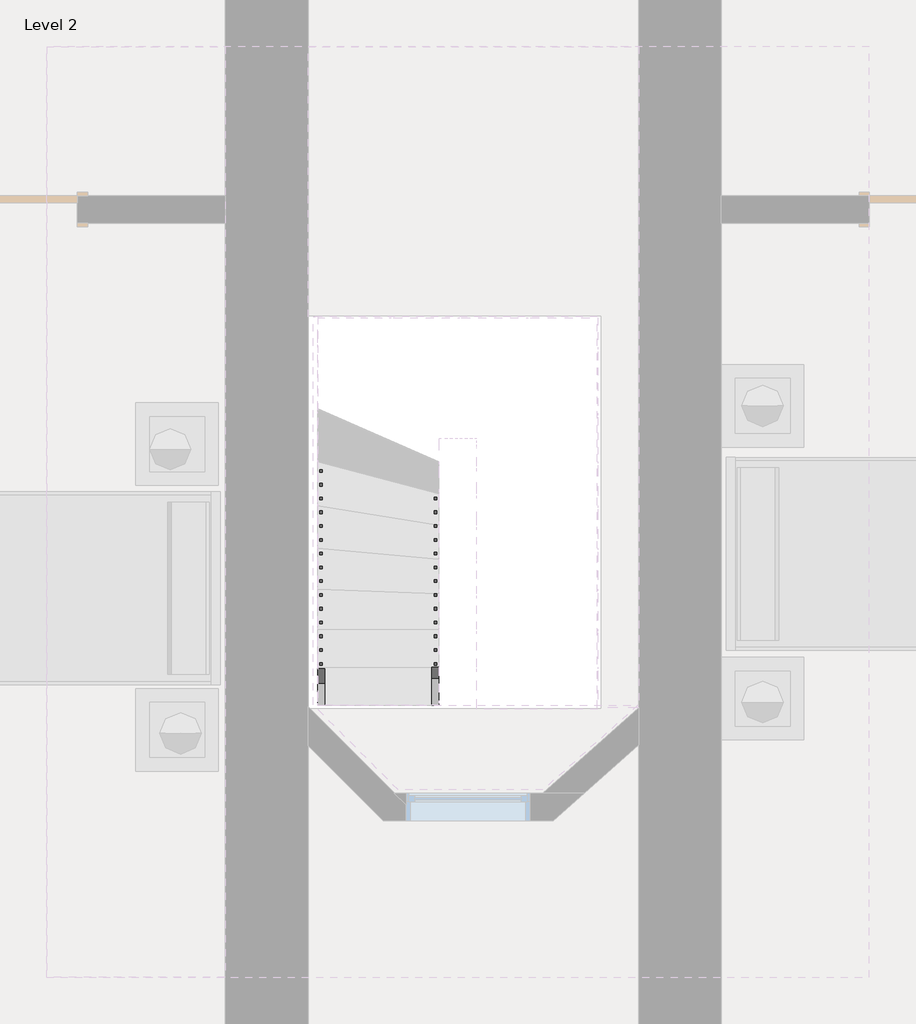
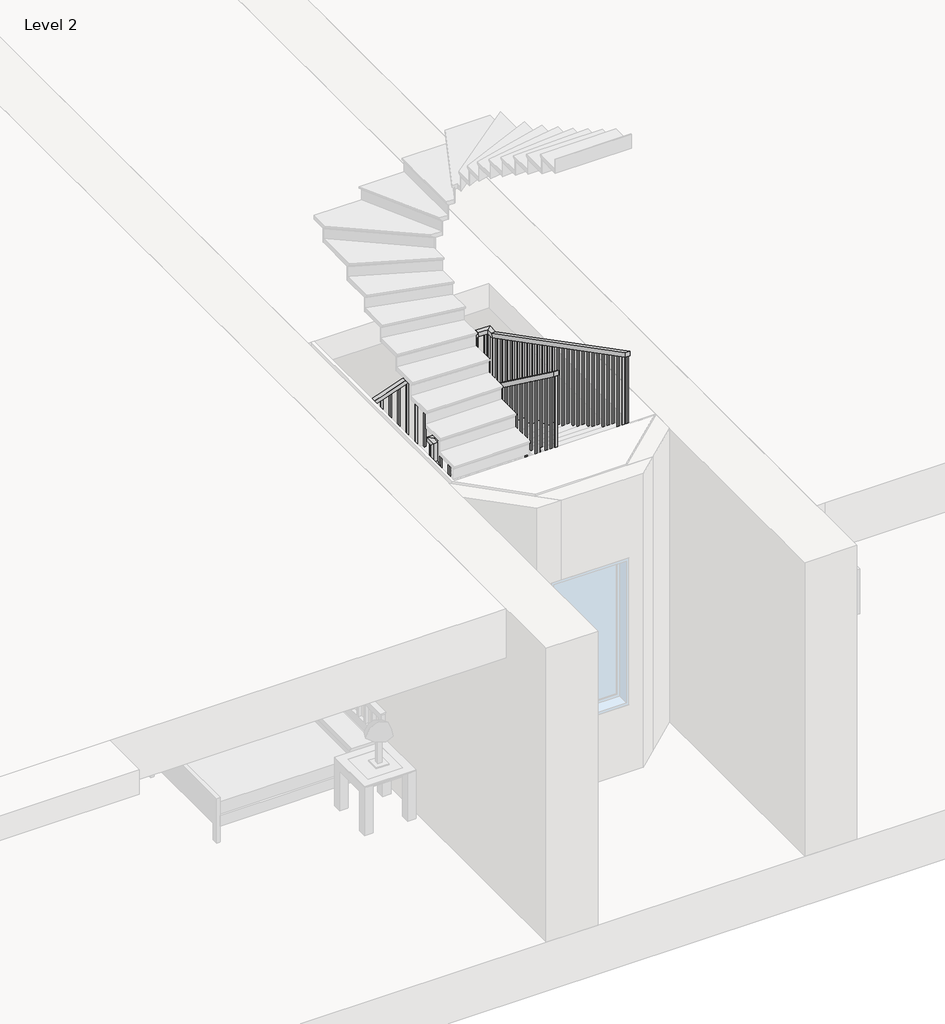
# One storey, part 4 of 5: 2 railings.
"""IFC4 building model written with IfcOpenShell, lengths in millimetres."""

from ifc_helpers import new_model, si_unit, frame, origin, place, context, project, spatial, polyline, outline, extrude, faceted_brep, element, save

model = new_model("IFC4")

# Units and contexts
model_context = context("Model", 3, world=origin())
ifc_project = project(units=[si_unit("LENGTHUNIT", "METRE", prefix="MILLI")], contexts=[model_context])

# Site, building, storey
site = spatial("IfcSite", under=ifc_project)
building = spatial("IfcBuilding", under=site)
storey = spatial("IfcBuildingStorey", under=building, Name="Level 2", Elevation=3657.6)

# Railings
placement = place(None, origin())
element("IfcRailing", 1, ObjectType="Handrail - Rectangular", at=placement, inside=storey, context=model_context, shape_type="SolidModel", body=[
    faceted_brep([(-5097.9987704, -4554.2130548, 4714.7238292), (-5097.9987704, -4554.2130548, 4651.6500708), (-5047.1987704, -4554.2130548, 4651.6500708), (-5047.1987704, -4554.2130548, 4714.7238292), (-5097.9987704, -2667.0424524, 6103.5505468), (-5097.9987704, -2616.2424524, 6077.8620662), (-5047.1987704, -2616.2424524, 6077.8620662), (-5047.1987704, -2667.0424524, 6103.5505468), (-5097.9987704, -2667.0424524, 6336.5326223), (-5097.9987704, -2616.2424524, 6285.7326223), (-5047.1987704, -2616.2424524, 6285.7326223), (-5047.1987704, -2667.0424524, 6336.5326223), (-5097.9987704, -2540.0424524, 6336.5326223), (-5097.9987704, -2540.0424524, 6285.7326223), (-5047.1987704, -2590.8424524, 6285.7326223), (-5047.1987704, -2590.8424524, 6336.5326223), (-4970.9987704, -2540.0424524, 6336.5326223), (-4937.2220362, -2540.0424524, 6285.7326223), (-4937.2220362, -2590.8424524, 6285.7326223), (-4970.9987704, -2590.8424524, 6336.5326223), (-4767.7987704, -2540.0424524, 6820.8625168), (-4767.7987704, -2590.8424524, 6820.8625168), (-4767.7987704, -2590.8424524, 6689.5552229), (-4767.7987704, -2540.0424524, 6689.5552229)], [[[0, 1, 2, 3]], [[1, 0, 4, 5]], [[2, 1, 5, 6]], [[3, 2, 6, 7]], [[0, 3, 7, 4]], [[5, 4, 8, 9]], [[6, 5, 9, 10]], [[7, 6, 10, 11]], [[4, 7, 11, 8]], [[9, 8, 12, 13]], [[10, 9, 13, 14]], [[11, 10, 14, 15]], [[8, 11, 15, 12]], [[13, 12, 16, 17]], [[14, 13, 17, 18]], [[15, 14, 18, 19]], [[12, 15, 19, 16]], [[20, 21, 22, 23]], [[17, 16, 20, 23]], [[18, 17, 23, 22]], [[19, 18, 22, 21]], [[16, 19, 21, 20]]]),
    faceted_brep([(-4716.9987704, -2540.0424524, 6839.4270399), (-4716.9987704, -2540.0424524, 6788.6270399), (-4767.7987704, -2540.0424524, 6788.6270399), (-4767.7987704, -2540.0424524, 6839.4270399), (-4716.9987704, -2622.481404, 6839.4270399), (-4716.9987704, -2639.1592773, 6788.6270399), (-4767.7987704, -2639.1592773, 6788.6270399), (-4767.7987704, -2622.481404, 6839.4270399), (-4716.9987704, -4554.2130546, 8261.0475994), (-4767.7987704, -4554.2130546, 8261.0475994), (-4767.7987704, -4554.2130546, 8197.973841), (-4716.9987704, -4554.2130546, 8197.973841)], [[[0, 1, 2, 3]], [[1, 0, 4, 5]], [[2, 1, 5, 6]], [[3, 2, 6, 7]], [[0, 3, 7, 4]], [[8, 9, 10, 11]], [[5, 4, 8, 11]], [[6, 5, 11, 10]], [[7, 6, 10, 9]], [[4, 7, 9, 8]]]),
    extrude(outline(polyline([(-4562.406404, 8204.0035782), (-4543.356404, 8189.984099), (-4543.356404, 7141.0285714), (-4562.406404, 7141.0285714), (-4562.406404, 8204.0035782)])), frame((-4751.9237704, 0.0, 0.0), z_axis=(1.0, 0.0, 0.0), x_axis=(0.0, 1.0, 0.0)), (0.0, 0.0, 1.0), 19.05),
    extrude(outline(polyline([(-4460.806404, 8129.2330225), (-4441.756404, 8115.2135433), (-4441.756404, 7141.0285714), (-4460.806404, 7141.0285714), (-4460.806404, 8129.2330225)])), frame((-4751.9237704, 0.0, 0.0), z_axis=(1.0, 0.0, 0.0), x_axis=(0.0, 1.0, 0.0)), (0.0, 0.0, 1.0), 19.05),
    extrude(outline(polyline([(-4359.206404, 8054.4624669), (-4340.156404, 8040.4429877), (-4340.156404, 7141.0285714), (-4359.206404, 7141.0285714), (-4359.206404, 8054.4624669)])), frame((-4751.9237704, 0.0, 0.0), z_axis=(1.0, 0.0, 0.0), x_axis=(0.0, 1.0, 0.0)), (0.0, 0.0, 1.0), 19.05),
    extrude(outline(polyline([(-4257.606404, 7979.6919113), (-4238.556404, 7965.6724321), (-4238.556404, 6966.8571429), (-4257.606404, 6966.8571429), (-4257.606404, 7979.6919113)])), frame((-4751.9237704, 0.0, 0.0), z_axis=(1.0, 0.0, 0.0), x_axis=(0.0, 1.0, 0.0)), (0.0, 0.0, 1.0), 19.05),
    extrude(outline(polyline([(-4156.006404, 7904.9213556), (-4136.956404, 7890.9018764), (-4136.956404, 6966.8571429), (-4156.006404, 6966.8571429), (-4156.006404, 7904.9213556)])), frame((-4751.9237704, 0.0, 0.0), z_axis=(1.0, 0.0, 0.0), x_axis=(0.0, 1.0, 0.0)), (0.0, 0.0, 1.0), 19.05),
    extrude(outline(polyline([(-4054.406404, 7830.1508), (-4035.356404, 7816.1313208), (-4035.356404, 6966.8571429), (-4054.406404, 6966.8571429), (-4054.406404, 7830.1508)])), frame((-4751.9237704, 0.0, 0.0), z_axis=(1.0, 0.0, 0.0), x_axis=(0.0, 1.0, 0.0)), (0.0, 0.0, 1.0), 19.05),
    extrude(outline(polyline([(-3952.806404, 7755.3802444), (-3933.756404, 7741.3607652), (-3933.756404, 6792.6857143), (-3952.806404, 6792.6857143), (-3952.806404, 7755.3802444)])), frame((-4751.9237704, 0.0, 0.0), z_axis=(1.0, 0.0, 0.0), x_axis=(0.0, 1.0, 0.0)), (0.0, 0.0, 1.0), 19.05),
    extrude(outline(polyline([(-3851.206404, 7680.6096887), (-3832.156404, 7666.5902095), (-3832.156404, 6792.6857143), (-3851.206404, 6792.6857143), (-3851.206404, 7680.6096887)])), frame((-4751.9237704, 0.0, 0.0), z_axis=(1.0, 0.0, 0.0), x_axis=(0.0, 1.0, 0.0)), (0.0, 0.0, 1.0), 19.05),
    extrude(outline(polyline([(-3749.606404, 7605.8391331), (-3730.556404, 7591.8196539), (-3730.556404, 6792.6857143), (-3749.606404, 6792.6857143), (-3749.606404, 7605.8391331)])), frame((-4751.9237704, 0.0, 0.0), z_axis=(1.0, 0.0, 0.0), x_axis=(0.0, 1.0, 0.0)), (0.0, 0.0, 1.0), 19.05),
    extrude(outline(polyline([(-3648.006404, 7531.0685775), (-3628.956404, 7517.0490983), (-3628.956404, 6618.5142857), (-3648.006404, 6618.5142857), (-3648.006404, 7531.0685775)])), frame((-4751.9237704, 0.0, 0.0), z_axis=(1.0, 0.0, 0.0), x_axis=(0.0, 1.0, 0.0)), (0.0, 0.0, 1.0), 19.05),
    extrude(outline(polyline([(-3546.406404, 7456.2980218), (-3527.356404, 7442.2785426), (-3527.356404, 6618.5142857), (-3546.406404, 6618.5142857), (-3546.406404, 7456.2980218)])), frame((-4751.9237704, 0.0, 0.0), z_axis=(1.0, 0.0, 0.0), x_axis=(0.0, 1.0, 0.0)), (0.0, 0.0, 1.0), 19.05),
    extrude(outline(polyline([(-3444.806404, 7381.5274662), (-3425.756404, 7367.507987), (-3425.756404, 6444.3428571), (-3444.806404, 6444.3428571), (-3444.806404, 7381.5274662)])), frame((-4751.9237704, 0.0, 0.0), z_axis=(1.0, 0.0, 0.0), x_axis=(0.0, 1.0, 0.0)), (0.0, 0.0, 1.0), 19.05),
    extrude(outline(polyline([(-3343.206404, 7306.7569106), (-3324.156404, 7292.7374314), (-3324.156404, 6444.3428571), (-3343.206404, 6444.3428571), (-3343.206404, 7306.7569106)])), frame((-4751.9237704, 0.0, 0.0), z_axis=(1.0, 0.0, 0.0), x_axis=(0.0, 1.0, 0.0)), (0.0, 0.0, 1.0), 19.05),
    extrude(outline(polyline([(-3241.606404, 7231.9863549), (-3222.556404, 7217.9668757), (-3222.556404, 6444.3428571), (-3241.606404, 6444.3428571), (-3241.606404, 7231.9863549)])), frame((-4751.9237704, 0.0, 0.0), z_axis=(1.0, 0.0, 0.0), x_axis=(0.0, 1.0, 0.0)), (0.0, 0.0, 1.0), 19.05),
    extrude(outline(polyline([(-3140.006404, 7157.2157993), (-3120.956404, 7143.1963201), (-3120.956404, 6270.1714286), (-3140.006404, 6270.1714286), (-3140.006404, 7157.2157993)])), frame((-4751.9237704, 0.0, 0.0), z_axis=(1.0, 0.0, 0.0), x_axis=(0.0, 1.0, 0.0)), (0.0, 0.0, 1.0), 19.05),
    extrude(outline(polyline([(-3038.406404, 7082.4452436), (-3019.356404, 7068.4257645), (-3019.356404, 6270.1714286), (-3038.406404, 6270.1714286), (-3038.406404, 7082.4452436)])), frame((-4751.9237704, 0.0, 0.0), z_axis=(1.0, 0.0, 0.0), x_axis=(0.0, 1.0, 0.0)), (0.0, 0.0, 1.0), 19.05),
    extrude(outline(polyline([(-2936.806404, 7007.674688), (-2917.756404, 6993.6552088), (-2917.756404, 6096.0), (-2936.806404, 6096.0), (-2936.806404, 7007.674688)])), frame((-4751.9237704, 0.0, 0.0), z_axis=(1.0, 0.0, 0.0), x_axis=(0.0, 1.0, 0.0)), (0.0, 0.0, 1.0), 19.05),
    extrude(outline(polyline([(-2835.206404, 6932.9041324), (-2816.156404, 6918.8846532), (-2816.156404, 6096.0), (-2835.206404, 6096.0), (-2835.206404, 6932.9041324)])), frame((-4751.9237704, 0.0, 0.0), z_axis=(1.0, 0.0, 0.0), x_axis=(0.0, 1.0, 0.0)), (0.0, 0.0, 1.0), 19.05),
    extrude(outline(polyline([(-2733.606404, 6858.1335767), (-2714.556404, 6844.1140976), (-2714.556404, 5921.8285714), (-2733.606404, 5921.8285714), (-2733.606404, 6858.1335767)])), frame((-4751.9237704, 0.0, 0.0), z_axis=(1.0, 0.0, 0.0), x_axis=(0.0, 1.0, 0.0)), (0.0, 0.0, 1.0), 19.05),
    extrude(outline(polyline([(6512.0699532, -4842.2624928), (6466.6640255, -4861.3124928), (5573.4857143, -4861.3124928), (5573.4857143, -4842.2624928), (6512.0699532, -4842.2624928)])), frame((0.0, -2574.9674524, 0.0), z_axis=(0.0, 1.0, 0.0), x_axis=(0.0, 0.0, 1.0)), (0.0, 0.0, 1.0), 19.05),
    extrude(outline(polyline([(6269.9050059, -4943.8624928), (6224.4990783, -4962.9124928), (5399.3142857, -4962.9124928), (5399.3142857, -4943.8624928), (6269.9050059, -4943.8624928)])), frame((0.0, -2574.9674524, 0.0), z_axis=(0.0, 1.0, 0.0), x_axis=(0.0, 0.0, 1.0)), (0.0, 0.0, 1.0), 19.05),
    extrude(outline(polyline([(-2633.3380548, 6065.2808881), (-2614.2880548, 6079.3003673), (-2614.2880548, 5050.9714286), (-2633.3380548, 5050.9714286), (-2633.3380548, 6065.2808881)])), frame((-5082.1237704, 0.0, 0.0), z_axis=(1.0, 0.0, 0.0), x_axis=(0.0, 1.0, 0.0)), (0.0, 0.0, 1.0), 19.05),
    extrude(outline(polyline([(-2734.9380548, 5990.5103325), (-2715.8880548, 6004.5298117), (-2715.8880548, 5050.9714286), (-2734.9380548, 5050.9714286), (-2734.9380548, 5990.5103325)])), frame((-5082.1237704, 0.0, 0.0), z_axis=(1.0, 0.0, 0.0), x_axis=(0.0, 1.0, 0.0)), (0.0, 0.0, 1.0), 19.05),
    extrude(outline(polyline([(-2836.5380548, 5915.7397768), (-2817.4880548, 5929.759256), (-2817.4880548, 4876.8), (-2836.5380548, 4876.8), (-2836.5380548, 5915.7397768)])), frame((-5082.1237704, 0.0, 0.0), z_axis=(1.0, 0.0, 0.0), x_axis=(0.0, 1.0, 0.0)), (0.0, 0.0, 1.0), 19.05),
    extrude(outline(polyline([(-2938.1380548, 5840.9692212), (-2919.0880548, 5854.9887004), (-2919.0880548, 4876.8), (-2938.1380548, 4876.8), (-2938.1380548, 5840.9692212)])), frame((-5082.1237704, 0.0, 0.0), z_axis=(1.0, 0.0, 0.0), x_axis=(0.0, 1.0, 0.0)), (0.0, 0.0, 1.0), 19.05),
    extrude(outline(polyline([(-3039.7380548, 5766.1986656), (-3020.6880548, 5780.2181448), (-3020.6880548, 4702.6285714), (-3039.7380548, 4702.6285714), (-3039.7380548, 5766.1986656)])), frame((-5082.1237704, 0.0, 0.0), z_axis=(1.0, 0.0, 0.0), x_axis=(0.0, 1.0, 0.0)), (0.0, 0.0, 1.0), 19.05),
    extrude(outline(polyline([(-3141.3380548, 5691.42811), (-3122.2880548, 5705.4475891), (-3122.2880548, 4702.6285714), (-3141.3380548, 4702.6285714), (-3141.3380548, 5691.42811)])), frame((-5082.1237704, 0.0, 0.0), z_axis=(1.0, 0.0, 0.0), x_axis=(0.0, 1.0, 0.0)), (0.0, 0.0, 1.0), 19.05),
    extrude(outline(polyline([(-3242.9380548, 5616.6575543), (-3223.8880548, 5630.6770335), (-3223.8880548, 4528.4571429), (-3242.9380548, 4528.4571429), (-3242.9380548, 5616.6575543)])), frame((-5082.1237704, 0.0, 0.0), z_axis=(1.0, 0.0, 0.0), x_axis=(0.0, 1.0, 0.0)), (0.0, 0.0, 1.0), 19.05),
    extrude(outline(polyline([(-3344.5380548, 5541.8869987), (-3325.4880548, 5555.9064779), (-3325.4880548, 4528.4571429), (-3344.5380548, 4528.4571429), (-3344.5380548, 5541.8869987)])), frame((-5082.1237704, 0.0, 0.0), z_axis=(1.0, 0.0, 0.0), x_axis=(0.0, 1.0, 0.0)), (0.0, 0.0, 1.0), 19.05),
    extrude(outline(polyline([(-3446.1380548, 5467.1164431), (-3427.0880548, 5481.1359223), (-3427.0880548, 4528.4571429), (-3446.1380548, 4528.4571429), (-3446.1380548, 5467.1164431)])), frame((-5082.1237704, 0.0, 0.0), z_axis=(1.0, 0.0, 0.0), x_axis=(0.0, 1.0, 0.0)), (0.0, 0.0, 1.0), 19.05),
    extrude(outline(polyline([(-3547.7380548, 5392.3458875), (-3528.6880548, 5406.3653666), (-3528.6880548, 4354.2857143), (-3547.7380548, 4354.2857143), (-3547.7380548, 5392.3458875)])), frame((-5082.1237704, 0.0, 0.0), z_axis=(1.0, 0.0, 0.0), x_axis=(0.0, 1.0, 0.0)), (0.0, 0.0, 1.0), 19.05),
    extrude(outline(polyline([(-3649.3380548, 5317.5753318), (-3630.2880548, 5331.594811), (-3630.2880548, 4354.2857143), (-3649.3380548, 4354.2857143), (-3649.3380548, 5317.5753318)])), frame((-5082.1237704, 0.0, 0.0), z_axis=(1.0, 0.0, 0.0), x_axis=(0.0, 1.0, 0.0)), (0.0, 0.0, 1.0), 19.05),
    extrude(outline(polyline([(-3750.9380548, 5242.8047762), (-3731.8880548, 5256.8242554), (-3731.8880548, 4180.1142857), (-3750.9380548, 4180.1142857), (-3750.9380548, 5242.8047762)])), frame((-5082.1237704, 0.0, 0.0), z_axis=(1.0, 0.0, 0.0), x_axis=(0.0, 1.0, 0.0)), (0.0, 0.0, 1.0), 19.05),
    extrude(outline(polyline([(-3852.5380548, 5168.0342206), (-3833.4880548, 5182.0536998), (-3833.4880548, 4180.1142857), (-3852.5380548, 4180.1142857), (-3852.5380548, 5168.0342206)])), frame((-5082.1237704, 0.0, 0.0), z_axis=(1.0, 0.0, 0.0), x_axis=(0.0, 1.0, 0.0)), (0.0, 0.0, 1.0), 19.05),
    extrude(outline(polyline([(-3954.1380548, 5093.263665), (-3935.0880548, 5107.2831441), (-3935.0880548, 4180.1142857), (-3954.1380548, 4180.1142857), (-3954.1380548, 5093.263665)])), frame((-5082.1237704, 0.0, 0.0), z_axis=(1.0, 0.0, 0.0), x_axis=(0.0, 1.0, 0.0)), (0.0, 0.0, 1.0), 19.05),
    extrude(outline(polyline([(-4055.7380548, 5018.4931093), (-4036.6880548, 5032.5125885), (-4036.6880548, 4005.9428571), (-4055.7380548, 4005.9428571), (-4055.7380548, 5018.4931093)])), frame((-5082.1237704, 0.0, 0.0), z_axis=(1.0, 0.0, 0.0), x_axis=(0.0, 1.0, 0.0)), (0.0, 0.0, 1.0), 19.05),
    extrude(outline(polyline([(-4157.3380548, 4943.7225537), (-4138.2880548, 4957.7420329), (-4138.2880548, 4005.9428571), (-4157.3380548, 4005.9428571), (-4157.3380548, 4943.7225537)])), frame((-5082.1237704, 0.0, 0.0), z_axis=(1.0, 0.0, 0.0), x_axis=(0.0, 1.0, 0.0)), (0.0, 0.0, 1.0), 19.05),
    extrude(outline(polyline([(-4258.9380548, 4868.9519981), (-4239.8880548, 4882.9714773), (-4239.8880548, 4005.9428571), (-4258.9380548, 4005.9428571), (-4258.9380548, 4868.9519981)])), frame((-5082.1237704, 0.0, 0.0), z_axis=(1.0, 0.0, 0.0), x_axis=(0.0, 1.0, 0.0)), (0.0, 0.0, 1.0), 19.05),
    extrude(outline(polyline([(-4360.5380548, 4794.1814424), (-4341.4880548, 4808.2009216), (-4341.4880548, 3831.7714286), (-4360.5380548, 3831.7714286), (-4360.5380548, 4794.1814424)])), frame((-5082.1237704, 0.0, 0.0), z_axis=(1.0, 0.0, 0.0), x_axis=(0.0, 1.0, 0.0)), (0.0, 0.0, 1.0), 19.05),
    extrude(outline(polyline([(-4462.1380548, 4719.4108868), (-4443.0880548, 4733.430366), (-4443.0880548, 3831.7714286), (-4462.1380548, 3831.7714286), (-4462.1380548, 4719.4108868)])), frame((-5082.1237704, 0.0, 0.0), z_axis=(1.0, 0.0, 0.0), x_axis=(0.0, 1.0, 0.0)), (0.0, 0.0, 1.0), 19.05),
    extrude(outline(polyline([(-4751.9237704, -2612.956404), (-4732.8737704, -2612.956404), (-4732.8737704, -2632.006404), (-4751.9237704, -2632.006404), (-4751.9237704, -2612.956404)])), frame((0.0, 0.0, 5921.8285714), z_axis=(0.0, 0.0, 1.0), x_axis=(1.0, 0.0, 0.0)), (0.0, 0.0, 1.0), 866.7984685),
    extrude(outline(polyline([(6772.7994235, -4732.8737704), (6727.3934959, -4751.9237704), (5747.6571429, -4751.9237704), (5747.6571429, -4732.8737704), (6772.7994235, -4732.8737704)])), frame((0.0, -2574.9674524, 0.0), z_axis=(0.0, 1.0, 0.0), x_axis=(0.0, 0.0, 1.0)), (0.0, 0.0, 1.0), 19.05),
    extrude(outline(polyline([(6730.8227099, -4750.485048), (6685.4167823, -4769.535048), (5747.6571429, -4769.535048), (5747.6571429, -4750.485048), (6730.8227099, -4750.485048)])), frame((0.0, -2574.9674524, 0.0), z_axis=(0.0, 1.0, 0.0), x_axis=(0.0, 0.0, 1.0)), (0.0, 0.0, 1.0), 19.05),
    extrude(outline(polyline([(-5064.5124928, -2574.9674524), (-5064.5124928, -2555.9174524), (-5045.4624928, -2555.9174524), (-5045.4624928, -2574.9674524), (-5064.5124928, -2574.9674524)])), frame((0.0, 0.0, 5225.1428571), z_axis=(0.0, 0.0, 1.0), x_axis=(1.0, 0.0, 0.0)), (0.0, 0.0, 1.0), 1060.5897652),
    extrude(outline(polyline([(-5063.0737704, -2574.9674524), (-5082.1237704, -2574.9674524), (-5082.1237704, -2555.9174524), (-5063.0737704, -2555.9174524), (-5063.0737704, -2574.9674524)])), frame((0.0, 0.0, 5225.1428571), z_axis=(0.0, 0.0, 1.0), x_axis=(1.0, 0.0, 0.0)), (0.0, 0.0, 1.0), 1060.5897652),
    extrude(outline(polyline([(-2632.006404, 6066.2608908), (-2612.956404, 6080.2803699), (-2612.956404, 5050.9714286), (-2632.006404, 5050.9714286), (-2632.006404, 6066.2608908)])), frame((-5082.1237704, 0.0, 0.0), z_axis=(1.0, 0.0, 0.0), x_axis=(0.0, 1.0, 0.0)), (0.0, 0.0, 1.0), 19.05),
    extrude(outline(polyline([(-4554.2130546, 8197.973841), (-4535.1630546, 8183.9543619), (-4535.1630546, 7141.0285714), (-4554.2130546, 7141.0285714), (-4554.2130546, 8197.973841)])), frame((-4751.9237704, 0.0, 0.0), z_axis=(1.0, 0.0, 0.0), x_axis=(0.0, 1.0, 0.0)), (0.0, 0.0, 1.0), 19.05),
    extrude(outline(polyline([(-4554.2130548, 4651.6500708), (-4535.1630548, 4665.66955), (-4535.1630548, 3831.7714286), (-4554.2130548, 3831.7714286), (-4554.2130548, 4651.6500708)])), frame((-5082.1237704, 0.0, 0.0), z_axis=(1.0, 0.0, 0.0), x_axis=(0.0, 1.0, 0.0)), (0.0, 0.0, 1.0), 19.05),
])
element("IfcRailing", 2, ObjectType="Handrail - Rectangular", at=placement, inside=storey, context=model_context, shape_type="SolidModel", body=[
    faceted_brep([(-5940.8822214, -4554.2130548, 4776.0197691), (-5940.8822214, -4554.2130548, 4718.8427889), (-5890.0822214, -4554.2130548, 4718.8427889), (-5890.0822214, -4554.2130548, 4776.0197691), (-5940.8822214, -1817.6237991, 6189.5953311), (-5940.8822214, -1805.2783851, 6138.7953311), (-5890.0822214, -1805.2783851, 6138.7953311), (-5890.0822214, -1817.6237991, 6189.5953311), (-5940.8822214, -1697.1590014, 6189.5953311), (-5940.8822214, -1697.1590014, 6138.7953311), (-5890.0822214, -1747.9590014, 6138.7953311), (-5890.0822214, -1747.9590014, 6189.5953311), (-5773.0008737, -1697.1590014, 6189.5953311), (-5764.4924766, -1697.1590014, 6138.7953311), (-5764.4924766, -1747.9590014, 6138.7953311), (-5773.0008737, -1747.9590014, 6189.5953311), (-4041.9966669, -1697.1590014, 6786.1760978), (-4033.4882698, -1697.1590014, 6735.3760978), (-4033.4882698, -1747.9590014, 6735.3760978), (-4041.9966669, -1747.9590014, 6786.1760978), (-3874.1153195, -1697.1590014, 6786.1760978), (-3874.1153195, -1697.1590014, 6735.3760978), (-3924.9153195, -1747.9590014, 6735.3760978), (-3924.9153195, -1747.9590014, 6786.1760978), (-3874.1153195, -1817.6237989, 6786.1760978), (-3874.1153195, -1829.9692129, 6735.3760978), (-3924.9153195, -1829.9692129, 6735.3760978), (-3924.9153195, -1817.6237989, 6786.1760978), (-3874.1153195, -4554.2130546, 8199.7516594), (-3924.9153195, -4554.2130546, 8199.7516594), (-3924.9153195, -4554.2130546, 8142.5746792), (-3874.1153195, -4554.2130546, 8142.5746792)], [[[0, 1, 2, 3]], [[1, 0, 4, 5]], [[2, 1, 5, 6]], [[3, 2, 6, 7]], [[0, 3, 7, 4]], [[5, 4, 8, 9]], [[6, 5, 9, 10]], [[7, 6, 10, 11]], [[4, 7, 11, 8]], [[9, 8, 12, 13]], [[10, 9, 13, 14]], [[11, 10, 14, 15]], [[8, 11, 15, 12]], [[13, 12, 16, 17]], [[14, 13, 17, 18]], [[15, 14, 18, 19]], [[12, 15, 19, 16]], [[17, 16, 20, 21]], [[18, 17, 21, 22]], [[19, 18, 22, 23]], [[16, 19, 23, 20]], [[21, 20, 24, 25]], [[22, 21, 25, 26]], [[23, 22, 26, 27]], [[20, 23, 27, 24]], [[28, 29, 30, 31]], [[25, 24, 28, 31]], [[26, 25, 31, 30]], [[27, 26, 30, 29]], [[24, 27, 29, 28]]]),
    extrude(outline(polyline([(-4449.6987989, 8088.5882078), (-4449.6987989, 7141.0285714), (-4468.7487989, 7141.0285714), (-4468.7487989, 8098.4284183), (-4449.6987989, 8088.5882078)])), frame((-3909.0403195, 0.0, 0.0), z_axis=(1.0, 0.0, 0.0), x_axis=(0.0, 1.0, 0.0)), (0.0, 0.0, 1.0), 19.05),
    extrude(outline(polyline([(-4348.0987989, 8036.1070849), (-4348.0987989, 7141.0285714), (-4367.1487989, 7141.0285714), (-4367.1487989, 8045.9472954), (-4348.0987989, 8036.1070849)])), frame((-3909.0403195, 0.0, 0.0), z_axis=(1.0, 0.0, 0.0), x_axis=(0.0, 1.0, 0.0)), (0.0, 0.0, 1.0), 19.05),
    extrude(outline(polyline([(-4246.4987989, 7983.625962), (-4246.4987989, 6966.8571429), (-4265.5487989, 6966.8571429), (-4265.5487989, 7993.4661725), (-4246.4987989, 7983.625962)])), frame((-3909.0403195, 0.0, 0.0), z_axis=(1.0, 0.0, 0.0), x_axis=(0.0, 1.0, 0.0)), (0.0, 0.0, 1.0), 19.05),
    extrude(outline(polyline([(-4144.8987989, 7931.1448391), (-4144.8987989, 6966.8571429), (-4163.9487989, 6966.8571429), (-4163.9487989, 7940.9850496), (-4144.8987989, 7931.1448391)])), frame((-3909.0403195, 0.0, 0.0), z_axis=(1.0, 0.0, 0.0), x_axis=(0.0, 1.0, 0.0)), (0.0, 0.0, 1.0), 19.05),
    extrude(outline(polyline([(-4043.2987989, 7878.6637162), (-4043.2987989, 6966.8571429), (-4062.3487989, 6966.8571429), (-4062.3487989, 7888.5039267), (-4043.2987989, 7878.6637162)])), frame((-3909.0403195, 0.0, 0.0), z_axis=(1.0, 0.0, 0.0), x_axis=(0.0, 1.0, 0.0)), (0.0, 0.0, 1.0), 19.05),
    extrude(outline(polyline([(-3941.6987989, 7826.1825933), (-3941.6987989, 6792.6857143), (-3960.7487989, 6792.6857143), (-3960.7487989, 7836.0228038), (-3941.6987989, 7826.1825933)])), frame((-3909.0403195, 0.0, 0.0), z_axis=(1.0, 0.0, 0.0), x_axis=(0.0, 1.0, 0.0)), (0.0, 0.0, 1.0), 19.05),
    extrude(outline(polyline([(-3840.0987989, 7773.7014704), (-3840.0987989, 6792.6857143), (-3859.1487989, 6792.6857143), (-3859.1487989, 7783.5416809), (-3840.0987989, 7773.7014704)])), frame((-3909.0403195, 0.0, 0.0), z_axis=(1.0, 0.0, 0.0), x_axis=(0.0, 1.0, 0.0)), (0.0, 0.0, 1.0), 19.05),
    extrude(outline(polyline([(-3738.4987989, 7721.2203475), (-3738.4987989, 6792.6857143), (-3757.5487989, 6792.6857143), (-3757.5487989, 7731.060558), (-3738.4987989, 7721.2203475)])), frame((-3909.0403195, 0.0, 0.0), z_axis=(1.0, 0.0, 0.0), x_axis=(0.0, 1.0, 0.0)), (0.0, 0.0, 1.0), 19.05),
    extrude(outline(polyline([(-3636.8987989, 7668.7392246), (-3636.8987989, 6618.5142857), (-3655.9487989, 6618.5142857), (-3655.9487989, 7678.5794351), (-3636.8987989, 7668.7392246)])), frame((-3909.0403195, 0.0, 0.0), z_axis=(1.0, 0.0, 0.0), x_axis=(0.0, 1.0, 0.0)), (0.0, 0.0, 1.0), 19.05),
    extrude(outline(polyline([(-3535.2987989, 7616.2581017), (-3535.2987989, 6618.5142857), (-3554.3487989, 6618.5142857), (-3554.3487989, 7626.0983122), (-3535.2987989, 7616.2581017)])), frame((-3909.0403195, 0.0, 0.0), z_axis=(1.0, 0.0, 0.0), x_axis=(0.0, 1.0, 0.0)), (0.0, 0.0, 1.0), 19.05),
    extrude(outline(polyline([(-3433.6987989, 7563.7769788), (-3433.6987989, 6618.5142857), (-3452.7487989, 6618.5142857), (-3452.7487989, 7573.6171893), (-3433.6987989, 7563.7769788)])), frame((-3909.0403195, 0.0, 0.0), z_axis=(1.0, 0.0, 0.0), x_axis=(0.0, 1.0, 0.0)), (0.0, 0.0, 1.0), 19.05),
    extrude(outline(polyline([(-3332.0987989, 7511.2958559), (-3332.0987989, 6444.3428571), (-3351.1487989, 6444.3428571), (-3351.1487989, 7521.1360664), (-3332.0987989, 7511.2958559)])), frame((-3909.0403195, 0.0, 0.0), z_axis=(1.0, 0.0, 0.0), x_axis=(0.0, 1.0, 0.0)), (0.0, 0.0, 1.0), 19.05),
    extrude(outline(polyline([(-3230.4987989, 7458.814733), (-3230.4987989, 6444.3428571), (-3249.5487989, 6444.3428571), (-3249.5487989, 7468.6549435), (-3230.4987989, 7458.814733)])), frame((-3909.0403195, 0.0, 0.0), z_axis=(1.0, 0.0, 0.0), x_axis=(0.0, 1.0, 0.0)), (0.0, 0.0, 1.0), 19.05),
    extrude(outline(polyline([(-3128.8987989, 7406.33361), (-3128.8987989, 6444.3428571), (-3147.9487989, 6444.3428571), (-3147.9487989, 7416.1738206), (-3128.8987989, 7406.33361)])), frame((-3909.0403195, 0.0, 0.0), z_axis=(1.0, 0.0, 0.0), x_axis=(0.0, 1.0, 0.0)), (0.0, 0.0, 1.0), 19.05),
    extrude(outline(polyline([(-3027.2987989, 7353.8524871), (-3027.2987989, 6270.1714286), (-3046.3487989, 6270.1714286), (-3046.3487989, 7363.6926977), (-3027.2987989, 7353.8524871)])), frame((-3909.0403195, 0.0, 0.0), z_axis=(1.0, 0.0, 0.0), x_axis=(0.0, 1.0, 0.0)), (0.0, 0.0, 1.0), 19.05),
    extrude(outline(polyline([(-2925.6987989, 7301.3713642), (-2925.6987989, 6270.1714286), (-2944.7487989, 6270.1714286), (-2944.7487989, 7311.2115748), (-2925.6987989, 7301.3713642)])), frame((-3909.0403195, 0.0, 0.0), z_axis=(1.0, 0.0, 0.0), x_axis=(0.0, 1.0, 0.0)), (0.0, 0.0, 1.0), 19.05),
    extrude(outline(polyline([(-2824.0987989, 7248.8902413), (-2824.0987989, 6270.1714286), (-2843.1487989, 6270.1714286), (-2843.1487989, 7258.7304519), (-2824.0987989, 7248.8902413)])), frame((-3909.0403195, 0.0, 0.0), z_axis=(1.0, 0.0, 0.0), x_axis=(0.0, 1.0, 0.0)), (0.0, 0.0, 1.0), 19.05),
    extrude(outline(polyline([(-2722.4987989, 7196.4091184), (-2722.4987989, 6096.0), (-2741.5487989, 6096.0), (-2741.5487989, 7206.249329), (-2722.4987989, 7196.4091184)])), frame((-3909.0403195, 0.0, 0.0), z_axis=(1.0, 0.0, 0.0), x_axis=(0.0, 1.0, 0.0)), (0.0, 0.0, 1.0), 19.05),
    extrude(outline(polyline([(-2620.8987989, 7143.9279955), (-2620.8987989, 6096.0), (-2639.9487989, 6096.0), (-2639.9487989, 7153.7682061), (-2620.8987989, 7143.9279955)])), frame((-3909.0403195, 0.0, 0.0), z_axis=(1.0, 0.0, 0.0), x_axis=(0.0, 1.0, 0.0)), (0.0, 0.0, 1.0), 19.05),
    extrude(outline(polyline([(-2519.2987989, 7091.4468726), (-2519.2987989, 6096.0), (-2538.3487989, 6096.0), (-2538.3487989, 7101.2870832), (-2519.2987989, 7091.4468726)])), frame((-3909.0403195, 0.0, 0.0), z_axis=(1.0, 0.0, 0.0), x_axis=(0.0, 1.0, 0.0)), (0.0, 0.0, 1.0), 19.05),
    extrude(outline(polyline([(-2417.6987989, 7038.9657497), (-2417.6987989, 6096.0), (-2436.7487989, 6096.0), (-2436.7487989, 7048.8059603), (-2417.6987989, 7038.9657497)])), frame((-3909.0403195, 0.0, 0.0), z_axis=(1.0, 0.0, 0.0), x_axis=(0.0, 1.0, 0.0)), (0.0, 0.0, 1.0), 19.05),
    extrude(outline(polyline([(-2316.0987989, 6986.4846268), (-2316.0987989, 5921.8285714), (-2335.1487989, 5921.8285714), (-2335.1487989, 6996.3248374), (-2316.0987989, 6986.4846268)])), frame((-3909.0403195, 0.0, 0.0), z_axis=(1.0, 0.0, 0.0), x_axis=(0.0, 1.0, 0.0)), (0.0, 0.0, 1.0), 19.05),
    extrude(outline(polyline([(-2214.4987989, 6934.0035039), (-2214.4987989, 5921.8285714), (-2233.5487989, 5921.8285714), (-2233.5487989, 6943.8437145), (-2214.4987989, 6934.0035039)])), frame((-3909.0403195, 0.0, 0.0), z_axis=(1.0, 0.0, 0.0), x_axis=(0.0, 1.0, 0.0)), (0.0, 0.0, 1.0), 19.05),
    extrude(outline(polyline([(-2112.8987989, 6881.522381), (-2112.8987989, 5921.8285714), (-2131.9487989, 5921.8285714), (-2131.9487989, 6891.3625916), (-2112.8987989, 6881.522381)])), frame((-3909.0403195, 0.0, 0.0), z_axis=(1.0, 0.0, 0.0), x_axis=(0.0, 1.0, 0.0)), (0.0, 0.0, 1.0), 19.05),
    extrude(outline(polyline([(-2011.2987989, 6829.0412581), (-2011.2987989, 5921.8285714), (-2030.3487989, 5921.8285714), (-2030.3487989, 6838.8814687), (-2011.2987989, 6829.0412581)])), frame((-3909.0403195, 0.0, 0.0), z_axis=(1.0, 0.0, 0.0), x_axis=(0.0, 1.0, 0.0)), (0.0, 0.0, 1.0), 19.05),
    extrude(outline(polyline([(-1909.6987989, 6776.5601352), (-1909.6987989, 5747.6571429), (-1928.7487989, 5747.6571429), (-1928.7487989, 6786.4003458), (-1909.6987989, 6776.5601352)])), frame((-3909.0403195, 0.0, 0.0), z_axis=(1.0, 0.0, 0.0), x_axis=(0.0, 1.0, 0.0)), (0.0, 0.0, 1.0), 19.05),
    extrude(outline(polyline([(-3949.9216669, -1713.0340014), (-3930.8716669, -1713.0340014), (-3930.8716669, -1732.0840014), (-3949.9216669, -1732.0840014), (-3949.9216669, -1713.0340014)])), frame((0.0, 0.0, 5747.6571429), z_axis=(0.0, 0.0, 1.0), x_axis=(1.0, 0.0, 0.0)), (0.0, 0.0, 1.0), 987.7189549),
    extrude(outline(polyline([(6727.8498917, -4055.3258737), (5747.6571429, -4055.3258737), (5747.6571429, -4036.2758737), (6734.415366, -4036.2758737), (6727.8498917, -4055.3258737)])), frame((0.0, -1732.0840014, 0.0), z_axis=(0.0, 1.0, 0.0), x_axis=(0.0, 0.0, 1.0)), (0.0, 0.0, 1.0), 19.05),
    extrude(outline(polyline([(6692.8340288, -4156.9258737), (5747.6571429, -4156.9258737), (5747.6571429, -4137.8758737), (6699.3995031, -4137.8758737), (6692.8340288, -4156.9258737)])), frame((0.0, -1732.0840014, 0.0), z_axis=(0.0, 1.0, 0.0), x_axis=(0.0, 0.0, 1.0)), (0.0, 0.0, 1.0), 19.05),
    extrude(outline(polyline([(6657.818166, -4258.5258737), (5747.6571429, -4258.5258737), (5747.6571429, -4239.4758737), (6664.3836403, -4239.4758737), (6657.818166, -4258.5258737)])), frame((0.0, -1732.0840014, 0.0), z_axis=(0.0, 1.0, 0.0), x_axis=(0.0, 0.0, 1.0)), (0.0, 0.0, 1.0), 19.05),
    extrude(outline(polyline([(6622.8023031, -4360.1258737), (5747.6571429, -4360.1258737), (5747.6571429, -4341.0758737), (6629.3677774, -4341.0758737), (6622.8023031, -4360.1258737)])), frame((0.0, -1732.0840014, 0.0), z_axis=(0.0, 1.0, 0.0), x_axis=(0.0, 0.0, 1.0)), (0.0, 0.0, 1.0), 19.05),
    extrude(outline(polyline([(6587.7864403, -4461.7258737), (5573.4857143, -4461.7258737), (5573.4857143, -4442.6758737), (6594.3519146, -4442.6758737), (6587.7864403, -4461.7258737)])), frame((0.0, -1732.0840014, 0.0), z_axis=(0.0, 1.0, 0.0), x_axis=(0.0, 0.0, 1.0)), (0.0, 0.0, 1.0), 19.05),
    extrude(outline(polyline([(6552.7705774, -4563.3258737), (5573.4857143, -4563.3258737), (5573.4857143, -4544.2758737), (6559.3360517, -4544.2758737), (6552.7705774, -4563.3258737)])), frame((0.0, -1732.0840014, 0.0), z_axis=(0.0, 1.0, 0.0), x_axis=(0.0, 0.0, 1.0)), (0.0, 0.0, 1.0), 19.05),
    extrude(outline(polyline([(6517.7547146, -4664.9258737), (5573.4857143, -4664.9258737), (5573.4857143, -4645.8758737), (6524.3201889, -4645.8758737), (6517.7547146, -4664.9258737)])), frame((0.0, -1732.0840014, 0.0), z_axis=(0.0, 1.0, 0.0), x_axis=(0.0, 0.0, 1.0)), (0.0, 0.0, 1.0), 19.05),
    extrude(outline(polyline([(6482.7388517, -4766.5258737), (5573.4857143, -4766.5258737), (5573.4857143, -4747.4758737), (6489.304326, -4747.4758737), (6482.7388517, -4766.5258737)])), frame((0.0, -1732.0840014, 0.0), z_axis=(0.0, 1.0, 0.0), x_axis=(0.0, 0.0, 1.0)), (0.0, 0.0, 1.0), 19.05),
    extrude(outline(polyline([(6447.7229889, -4868.1258737), (5573.4857143, -4868.1258737), (5573.4857143, -4849.0758737), (6454.2884632, -4849.0758737), (6447.7229889, -4868.1258737)])), frame((0.0, -1732.0840014, 0.0), z_axis=(0.0, 1.0, 0.0), x_axis=(0.0, 0.0, 1.0)), (0.0, 0.0, 1.0), 19.05),
    extrude(outline(polyline([(6412.707126, -4969.7258737), (5399.3142857, -4969.7258737), (5399.3142857, -4950.6758737), (6419.2726003, -4950.6758737), (6412.707126, -4969.7258737)])), frame((0.0, -1732.0840014, 0.0), z_axis=(0.0, 1.0, 0.0), x_axis=(0.0, 0.0, 1.0)), (0.0, 0.0, 1.0), 19.05),
    extrude(outline(polyline([(6377.6912632, -5071.3258737), (5399.3142857, -5071.3258737), (5399.3142857, -5052.2758737), (6384.2567375, -5052.2758737), (6377.6912632, -5071.3258737)])), frame((0.0, -1732.0840014, 0.0), z_axis=(0.0, 1.0, 0.0), x_axis=(0.0, 0.0, 1.0)), (0.0, 0.0, 1.0), 19.05),
    extrude(outline(polyline([(6342.6754003, -5172.9258737), (5399.3142857, -5172.9258737), (5399.3142857, -5153.8758737), (6349.2408746, -5153.8758737), (6342.6754003, -5172.9258737)])), frame((0.0, -1732.0840014, 0.0), z_axis=(0.0, 1.0, 0.0), x_axis=(0.0, 0.0, 1.0)), (0.0, 0.0, 1.0), 19.05),
    extrude(outline(polyline([(6307.6595375, -5274.5258737), (5399.3142857, -5274.5258737), (5399.3142857, -5255.4758737), (6314.2250118, -5255.4758737), (6307.6595375, -5274.5258737)])), frame((0.0, -1732.0840014, 0.0), z_axis=(0.0, 1.0, 0.0), x_axis=(0.0, 0.0, 1.0)), (0.0, 0.0, 1.0), 19.05),
    extrude(outline(polyline([(6272.6436746, -5376.1258737), (5399.3142857, -5376.1258737), (5399.3142857, -5357.0758737), (6279.2091489, -5357.0758737), (6272.6436746, -5376.1258737)])), frame((0.0, -1732.0840014, 0.0), z_axis=(0.0, 1.0, 0.0), x_axis=(0.0, 0.0, 1.0)), (0.0, 0.0, 1.0), 19.05),
    extrude(outline(polyline([(6237.6278118, -5477.7258737), (5225.1428571, -5477.7258737), (5225.1428571, -5458.6758737), (6244.1932861, -5458.6758737), (6237.6278118, -5477.7258737)])), frame((0.0, -1732.0840014, 0.0), z_axis=(0.0, 1.0, 0.0), x_axis=(0.0, 0.0, 1.0)), (0.0, 0.0, 1.0), 19.05),
    extrude(outline(polyline([(6202.6119489, -5579.3258737), (5225.1428571, -5579.3258737), (5225.1428571, -5560.2758737), (6209.1774232, -5560.2758737), (6202.6119489, -5579.3258737)])), frame((0.0, -1732.0840014, 0.0), z_axis=(0.0, 1.0, 0.0), x_axis=(0.0, 0.0, 1.0)), (0.0, 0.0, 1.0), 19.05),
    extrude(outline(polyline([(6167.5960861, -5680.9258737), (5225.1428571, -5680.9258737), (5225.1428571, -5661.8758737), (6174.1615604, -5661.8758737), (6167.5960861, -5680.9258737)])), frame((0.0, -1732.0840014, 0.0), z_axis=(0.0, 1.0, 0.0), x_axis=(0.0, 0.0, 1.0)), (0.0, 0.0, 1.0), 19.05),
    extrude(outline(polyline([(-5823.4072214, -1713.0340014), (-5804.3572214, -1713.0340014), (-5804.3572214, -1732.0840014), (-5823.4072214, -1732.0840014), (-5823.4072214, -1713.0340014)])), frame((0.0, 0.0, 5225.1428571), z_axis=(0.0, 0.0, 1.0), x_axis=(1.0, 0.0, 0.0)), (0.0, 0.0, 1.0), 913.6524739),
    extrude(outline(polyline([(-1903.0880548, 6088.2720899), (-1903.0880548, 5225.1428571), (-1922.1380548, 5225.1428571), (-1922.1380548, 6078.4318794), (-1903.0880548, 6088.2720899)])), frame((-5925.0072214, 0.0, 0.0), z_axis=(1.0, 0.0, 0.0), x_axis=(0.0, 1.0, 0.0)), (0.0, 0.0, 1.0), 19.05),
    extrude(outline(polyline([(-2004.6880548, 6035.790967), (-2004.6880548, 5050.9714286), (-2023.7380548, 5050.9714286), (-2023.7380548, 6025.9507565), (-2004.6880548, 6035.790967)])), frame((-5925.0072214, 0.0, 0.0), z_axis=(1.0, 0.0, 0.0), x_axis=(0.0, 1.0, 0.0)), (0.0, 0.0, 1.0), 19.05),
    extrude(outline(polyline([(-2106.2880548, 5983.3098441), (-2106.2880548, 5050.9714286), (-2125.3380548, 5050.9714286), (-2125.3380548, 5973.4696336), (-2106.2880548, 5983.3098441)])), frame((-5925.0072214, 0.0, 0.0), z_axis=(1.0, 0.0, 0.0), x_axis=(0.0, 1.0, 0.0)), (0.0, 0.0, 1.0), 19.05),
    extrude(outline(polyline([(-2207.8880548, 5930.8287212), (-2207.8880548, 5050.9714286), (-2226.9380548, 5050.9714286), (-2226.9380548, 5920.9885107), (-2207.8880548, 5930.8287212)])), frame((-5925.0072214, 0.0, 0.0), z_axis=(1.0, 0.0, 0.0), x_axis=(0.0, 1.0, 0.0)), (0.0, 0.0, 1.0), 19.05),
    extrude(outline(polyline([(-2309.4880548, 5878.3475983), (-2309.4880548, 5050.9714286), (-2328.5380548, 5050.9714286), (-2328.5380548, 5868.5073877), (-2309.4880548, 5878.3475983)])), frame((-5925.0072214, 0.0, 0.0), z_axis=(1.0, 0.0, 0.0), x_axis=(0.0, 1.0, 0.0)), (0.0, 0.0, 1.0), 19.05),
    extrude(outline(polyline([(-2411.0880548, 5825.8664754), (-2411.0880548, 4876.8), (-2430.1380548, 4876.8), (-2430.1380548, 5816.0262648), (-2411.0880548, 5825.8664754)])), frame((-5925.0072214, 0.0, 0.0), z_axis=(1.0, 0.0, 0.0), x_axis=(0.0, 1.0, 0.0)), (0.0, 0.0, 1.0), 19.05),
    extrude(outline(polyline([(-2512.6880548, 5773.3853525), (-2512.6880548, 4876.8), (-2531.7380548, 4876.8), (-2531.7380548, 5763.5451419), (-2512.6880548, 5773.3853525)])), frame((-5925.0072214, 0.0, 0.0), z_axis=(1.0, 0.0, 0.0), x_axis=(0.0, 1.0, 0.0)), (0.0, 0.0, 1.0), 19.05),
    extrude(outline(polyline([(-2614.2880548, 5720.9042295), (-2614.2880548, 4876.8), (-2633.3380548, 4876.8), (-2633.3380548, 5711.064019), (-2614.2880548, 5720.9042295)])), frame((-5925.0072214, 0.0, 0.0), z_axis=(1.0, 0.0, 0.0), x_axis=(0.0, 1.0, 0.0)), (0.0, 0.0, 1.0), 19.05),
    extrude(outline(polyline([(-2715.8880548, 5668.4231066), (-2715.8880548, 4876.8), (-2734.9380548, 4876.8), (-2734.9380548, 5658.5828961), (-2715.8880548, 5668.4231066)])), frame((-5925.0072214, 0.0, 0.0), z_axis=(1.0, 0.0, 0.0), x_axis=(0.0, 1.0, 0.0)), (0.0, 0.0, 1.0), 19.05),
    extrude(outline(polyline([(-2817.4880548, 5615.9419837), (-2817.4880548, 4702.6285714), (-2836.5380548, 4702.6285714), (-2836.5380548, 5606.1017732), (-2817.4880548, 5615.9419837)])), frame((-5925.0072214, 0.0, 0.0), z_axis=(1.0, 0.0, 0.0), x_axis=(0.0, 1.0, 0.0)), (0.0, 0.0, 1.0), 19.05),
    extrude(outline(polyline([(-2919.0880548, 5563.4608608), (-2919.0880548, 4702.6285714), (-2938.1380548, 4702.6285714), (-2938.1380548, 5553.6206503), (-2919.0880548, 5563.4608608)])), frame((-5925.0072214, 0.0, 0.0), z_axis=(1.0, 0.0, 0.0), x_axis=(0.0, 1.0, 0.0)), (0.0, 0.0, 1.0), 19.05),
    extrude(outline(polyline([(-3020.6880548, 5510.9797379), (-3020.6880548, 4702.6285714), (-3039.7380548, 4702.6285714), (-3039.7380548, 5501.1395273), (-3020.6880548, 5510.9797379)])), frame((-5925.0072214, 0.0, 0.0), z_axis=(1.0, 0.0, 0.0), x_axis=(0.0, 1.0, 0.0)), (0.0, 0.0, 1.0), 19.05),
    extrude(outline(polyline([(-3122.2880548, 5458.498615), (-3122.2880548, 4528.4571429), (-3141.3380548, 4528.4571429), (-3141.3380548, 5448.6584044), (-3122.2880548, 5458.498615)])), frame((-5925.0072214, 0.0, 0.0), z_axis=(1.0, 0.0, 0.0), x_axis=(0.0, 1.0, 0.0)), (0.0, 0.0, 1.0), 19.05),
    extrude(outline(polyline([(-3223.8880548, 5406.0174921), (-3223.8880548, 4528.4571429), (-3242.9380548, 4528.4571429), (-3242.9380548, 5396.1772815), (-3223.8880548, 5406.0174921)])), frame((-5925.0072214, 0.0, 0.0), z_axis=(1.0, 0.0, 0.0), x_axis=(0.0, 1.0, 0.0)), (0.0, 0.0, 1.0), 19.05),
    extrude(outline(polyline([(-3325.4880548, 5353.5363692), (-3325.4880548, 4528.4571429), (-3344.5380548, 4528.4571429), (-3344.5380548, 5343.6961586), (-3325.4880548, 5353.5363692)])), frame((-5925.0072214, 0.0, 0.0), z_axis=(1.0, 0.0, 0.0), x_axis=(0.0, 1.0, 0.0)), (0.0, 0.0, 1.0), 19.05),
    extrude(outline(polyline([(-3427.0880548, 5301.0552462), (-3427.0880548, 4354.2857143), (-3446.1380548, 4354.2857143), (-3446.1380548, 5291.2150357), (-3427.0880548, 5301.0552462)])), frame((-5925.0072214, 0.0, 0.0), z_axis=(1.0, 0.0, 0.0), x_axis=(0.0, 1.0, 0.0)), (0.0, 0.0, 1.0), 19.05),
    extrude(outline(polyline([(-3528.6880548, 5248.5741233), (-3528.6880548, 4354.2857143), (-3547.7380548, 4354.2857143), (-3547.7380548, 5238.7339128), (-3528.6880548, 5248.5741233)])), frame((-5925.0072214, 0.0, 0.0), z_axis=(1.0, 0.0, 0.0), x_axis=(0.0, 1.0, 0.0)), (0.0, 0.0, 1.0), 19.05),
    extrude(outline(polyline([(-3630.2880548, 5196.0930004), (-3630.2880548, 4354.2857143), (-3649.3380548, 4354.2857143), (-3649.3380548, 5186.2527899), (-3630.2880548, 5196.0930004)])), frame((-5925.0072214, 0.0, 0.0), z_axis=(1.0, 0.0, 0.0), x_axis=(0.0, 1.0, 0.0)), (0.0, 0.0, 1.0), 19.05),
    extrude(outline(polyline([(-3731.8880548, 5143.6118775), (-3731.8880548, 4180.1142857), (-3750.9380548, 4180.1142857), (-3750.9380548, 5133.771667), (-3731.8880548, 5143.6118775)])), frame((-5925.0072214, 0.0, 0.0), z_axis=(1.0, 0.0, 0.0), x_axis=(0.0, 1.0, 0.0)), (0.0, 0.0, 1.0), 19.05),
    extrude(outline(polyline([(-3833.4880548, 5091.1307546), (-3833.4880548, 4180.1142857), (-3852.5380548, 4180.1142857), (-3852.5380548, 5081.290544), (-3833.4880548, 5091.1307546)])), frame((-5925.0072214, 0.0, 0.0), z_axis=(1.0, 0.0, 0.0), x_axis=(0.0, 1.0, 0.0)), (0.0, 0.0, 1.0), 19.05),
    extrude(outline(polyline([(-3935.0880548, 5038.6496317), (-3935.0880548, 4180.1142857), (-3954.1380548, 4180.1142857), (-3954.1380548, 5028.8094211), (-3935.0880548, 5038.6496317)])), frame((-5925.0072214, 0.0, 0.0), z_axis=(1.0, 0.0, 0.0), x_axis=(0.0, 1.0, 0.0)), (0.0, 0.0, 1.0), 19.05),
    extrude(outline(polyline([(-4036.6880548, 4986.1685088), (-4036.6880548, 4005.9428571), (-4055.7380548, 4005.9428571), (-4055.7380548, 4976.3282982), (-4036.6880548, 4986.1685088)])), frame((-5925.0072214, 0.0, 0.0), z_axis=(1.0, 0.0, 0.0), x_axis=(0.0, 1.0, 0.0)), (0.0, 0.0, 1.0), 19.05),
    extrude(outline(polyline([(-4138.2880548, 4933.6873859), (-4138.2880548, 4005.9428571), (-4157.3380548, 4005.9428571), (-4157.3380548, 4923.8471753), (-4138.2880548, 4933.6873859)])), frame((-5925.0072214, 0.0, 0.0), z_axis=(1.0, 0.0, 0.0), x_axis=(0.0, 1.0, 0.0)), (0.0, 0.0, 1.0), 19.05),
    extrude(outline(polyline([(-4239.8880548, 4881.2062629), (-4239.8880548, 4005.9428571), (-4258.9380548, 4005.9428571), (-4258.9380548, 4871.3660524), (-4239.8880548, 4881.2062629)])), frame((-5925.0072214, 0.0, 0.0), z_axis=(1.0, 0.0, 0.0), x_axis=(0.0, 1.0, 0.0)), (0.0, 0.0, 1.0), 19.05),
    extrude(outline(polyline([(-4341.4880548, 4828.72514), (-4341.4880548, 3831.7714286), (-4360.5380548, 3831.7714286), (-4360.5380548, 4818.8849295), (-4341.4880548, 4828.72514)])), frame((-5925.0072214, 0.0, 0.0), z_axis=(1.0, 0.0, 0.0), x_axis=(0.0, 1.0, 0.0)), (0.0, 0.0, 1.0), 19.05),
    extrude(outline(polyline([(-4443.0880548, 4776.2440171), (-4443.0880548, 3831.7714286), (-4462.1380548, 3831.7714286), (-4462.1380548, 4766.4038066), (-4443.0880548, 4776.2440171)])), frame((-5925.0072214, 0.0, 0.0), z_axis=(1.0, 0.0, 0.0), x_axis=(0.0, 1.0, 0.0)), (0.0, 0.0, 1.0), 19.05),
    extrude(outline(polyline([(-3889.9903195, -1808.0987989), (-3889.9903195, -1827.1487989), (-3909.0403195, -1827.1487989), (-3909.0403195, -1808.0987989), (-3889.9903195, -1808.0987989)])), frame((0.0, 0.0, 5747.6571429), z_axis=(0.0, 0.0, 1.0), x_axis=(1.0, 0.0, 0.0)), (0.0, 0.0, 1.0), 987.7189549),
    extrude(outline(polyline([(-3909.0403195, -1713.0340014), (-3889.9903195, -1713.0340014), (-3889.9903195, -1732.0840014), (-3909.0403195, -1732.0840014), (-3909.0403195, -1713.0340014)])), frame((0.0, 0.0, 5747.6571429), z_axis=(0.0, 0.0, 1.0), x_axis=(1.0, 0.0, 0.0)), (0.0, 0.0, 1.0), 987.7189549),
    extrude(outline(polyline([(6729.1609899, -4051.5216669), (5747.6571429, -4051.5216669), (5747.6571429, -4032.4716669), (6735.7264642, -4032.4716669), (6729.1609899, -4051.5216669)])), frame((0.0, -1732.0840014, 0.0), z_axis=(0.0, 1.0, 0.0), x_axis=(0.0, 0.0, 1.0)), (0.0, 0.0, 1.0), 19.05),
    extrude(outline(polyline([(-5782.5258737, -1713.0340014), (-5763.4758737, -1713.0340014), (-5763.4758737, -1732.0840014), (-5782.5258737, -1732.0840014), (-5782.5258737, -1713.0340014)])), frame((0.0, 0.0, 5225.1428571), z_axis=(0.0, 0.0, 1.0), x_axis=(1.0, 0.0, 0.0)), (0.0, 0.0, 1.0), 913.6524739),
    extrude(outline(polyline([(-5925.0072214, -1732.0840014), (-5925.0072214, -1713.0340014), (-5905.9572214, -1713.0340014), (-5905.9572214, -1732.0840014), (-5925.0072214, -1732.0840014)])), frame((0.0, 0.0, 5225.1428571), z_axis=(0.0, 0.0, 1.0), x_axis=(1.0, 0.0, 0.0)), (0.0, 0.0, 1.0), 913.6524739),
    extrude(outline(polyline([(-1808.0987991, 6137.3384561), (-1808.0987991, 5225.1428571), (-1827.1487991, 5225.1428571), (-1827.1487991, 6127.4982456), (-1808.0987991, 6137.3384561)])), frame((-5925.0072214, 0.0, 0.0), z_axis=(1.0, 0.0, 0.0), x_axis=(0.0, 1.0, 0.0)), (0.0, 0.0, 1.0), 19.05),
    extrude(outline(polyline([(-4535.1630546, 8132.7344687), (-4535.1630546, 7141.0285714), (-4554.2130546, 7141.0285714), (-4554.2130546, 8142.5746792), (-4535.1630546, 8132.7344687)])), frame((-3909.0403195, 0.0, 0.0), z_axis=(1.0, 0.0, 0.0), x_axis=(0.0, 1.0, 0.0)), (0.0, 0.0, 1.0), 19.05),
    extrude(outline(polyline([(-4535.1630548, 4728.6829995), (-4535.1630548, 3831.7714286), (-4554.2130548, 3831.7714286), (-4554.2130548, 4718.8427889), (-4535.1630548, 4728.6829995)])), frame((-5925.0072214, 0.0, 0.0), z_axis=(1.0, 0.0, 0.0), x_axis=(0.0, 1.0, 0.0)), (0.0, 0.0, 1.0), 19.05),
])

save(model, "model.ifc")

# Revit data of these elements
# Type "Handrail - Rectangular"
#   Assembly Code = "C2010400"
#   built-in parameter 1008612 = 0.0416667 (stored number, unit not read)
#   built-in parameter 1008611 = 0.0416667 (stored number, unit not read)
#   built-in parameter 1008609 = 0.333333 (stored number, unit not read)
#   built-in parameter 1008604 = 0.166667 (stored number, unit not read)
#   built-in parameter 1008603 = 0.166667 (stored number, unit not read)
#   Railing Height = 3' - 0"
#   built-in parameter 1008630 = 2
#   built-in parameter 1008610 = 2
#   built-in parameter 1008618 = Baluster - Square : 3/4"
# Elements 1, 2 (IfcRailing, "Handrail - Rectangular")
#   Phase Created = New Construction
